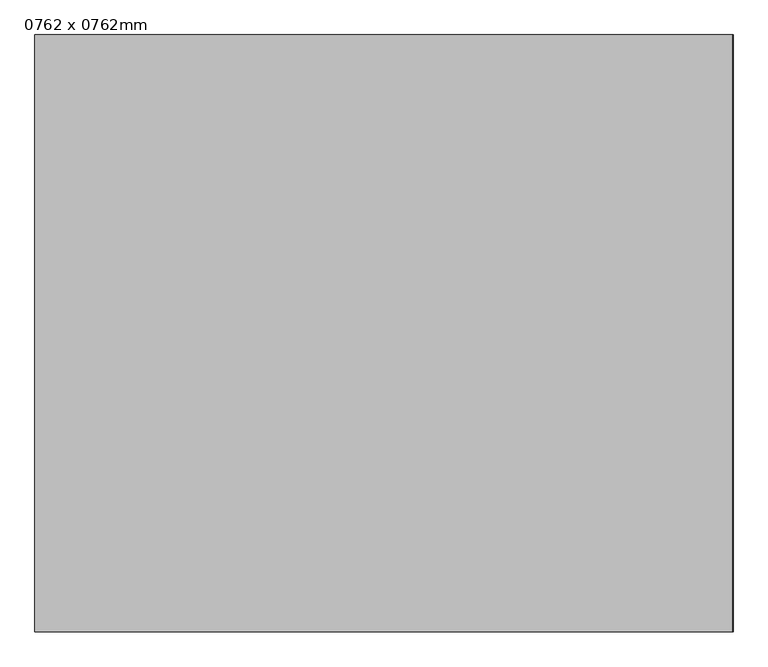
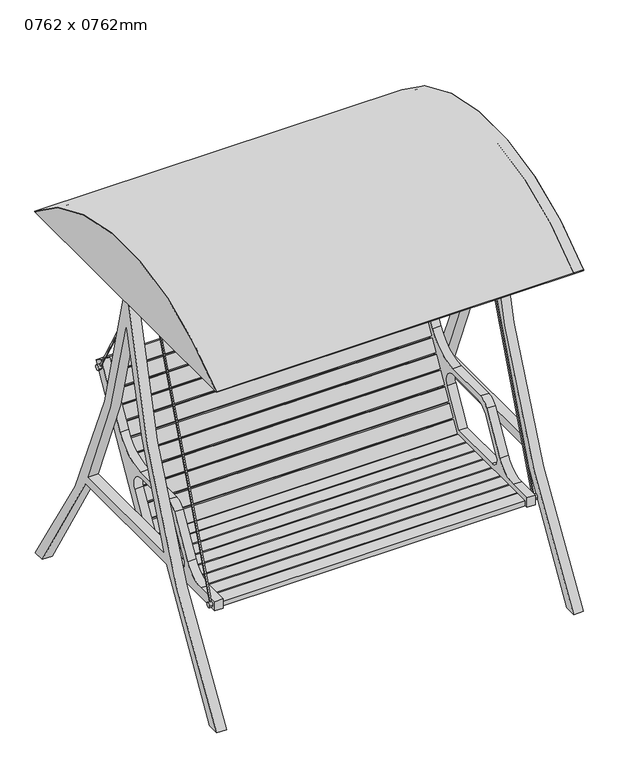
"""IFC4 building model written with IfcOpenShell, lengths in millimetres: furniture geometry, 0762 x 0762mm."""

from ifc_helpers import new_model, si_unit, point, frame, frame_2d, origin, place, context, project, spatial, polyline, circle_curve, trimmed, segment, composite_curve, outline, extrude, source, transform, mapped, element, save


def furniture_0762_x_0762mm_a8fad5e2(model_context):
    return source(origin(), model_context, "Body", "SweptSolid", [
        extrude(outline(composite_curve([segment(trimmed(circle_curve(frame_2d((4189.9023331, 1950.2809332)), 3303.1244251), [point((933.45, 1396.9734505))], [point((1524.0, 0.0))], True, "CARTESIAN"), True, "CONTINUOUS"), segment(polyline([(1524.0, 0.0), (1476.936255, 0.0)]), True, "CONTINUOUS"), segment(trimmed(circle_curve(frame_2d((4189.9023331, 1950.2809332)), 3341.2244251), [point((1476.936255, 0.0))], [point((1186.3373595, 486.5944542))], False, "CARTESIAN"), True, "CONTINUOUS"), segment(polyline([(1186.3373595, 486.5944542), (642.4626405, 486.5944542)]), True, "CONTINUOUS"), segment(trimmed(circle_curve(frame_2d((-2361.1023331, 1950.2809332)), 3341.2244251), [point((642.4626405, 486.5944542))], [point((351.863745, 0.0))], False, "CARTESIAN"), True, "CONTINUOUS"), segment(polyline([(351.863745, 0.0), (304.8, 0.0)]), True, "CONTINUOUS"), segment(trimmed(circle_curve(frame_2d((-2361.1023331, 1950.2809332)), 3303.1244251), [point((304.8, 0.0))], [point((895.35, 1396.9734505))], True, "CARTESIAN"), True, "CONTINUOUS"), segment(polyline([(895.35, 1396.9734505), (895.35, 1524.0), (914.4, 1524.0), (933.45, 1524.0), (933.45, 1396.9734505)]), True, "CONTINUOUS")], self_intersect=False), holes=[composite_curve([segment(polyline([(660.7321842, 524.6944542), (1168.0678158, 524.6944542)]), True, "CONTINUOUS"), segment(trimmed(circle_curve(frame_2d((4189.9023331, 1950.2809332)), 3341.2244251), [point((1168.0678158, 524.6944542))], [point((914.4, 1290.8378915))], False, "CARTESIAN"), True, "CONTINUOUS"), segment(trimmed(circle_curve(frame_2d((-2361.1023331, 1950.2809332)), 3341.2244251), [point((914.4, 1290.8378915))], [point((660.7321842, 524.6944542))], False, "CARTESIAN"), True, "CONTINUOUS")], self_intersect=False)]), frame((-272.362745, 0.0, 0.0), z_axis=(1.0, 0.0, 0.0), x_axis=(0.0, 1.0, 0.0)), (0.0, 0.0, 1.0), 38.1),
        extrude(outline(composite_curve([segment(trimmed(circle_curve(frame_2d((4189.9023331, 1950.2809332)), 3303.1244251), [point((933.45, 1396.9734505))], [point((1524.0, 0.0))], True, "CARTESIAN"), True, "CONTINUOUS"), segment(polyline([(1524.0, 0.0), (1476.936255, 0.0)]), True, "CONTINUOUS"), segment(trimmed(circle_curve(frame_2d((4189.9023331, 1950.2809332)), 3341.2244251), [point((1476.936255, 0.0))], [point((1186.3373595, 486.5944542))], False, "CARTESIAN"), True, "CONTINUOUS"), segment(polyline([(1186.3373595, 486.5944542), (642.4626405, 486.5944542)]), True, "CONTINUOUS"), segment(trimmed(circle_curve(frame_2d((-2361.1023331, 1950.2809332)), 3341.2244251), [point((642.4626405, 486.5944542))], [point((351.863745, 0.0))], False, "CARTESIAN"), True, "CONTINUOUS"), segment(polyline([(351.863745, 0.0), (304.8, 0.0)]), True, "CONTINUOUS"), segment(trimmed(circle_curve(frame_2d((-2361.1023331, 1950.2809332)), 3303.1244251), [point((304.8, 0.0))], [point((895.35, 1396.9734505))], True, "CARTESIAN"), True, "CONTINUOUS"), segment(polyline([(895.35, 1396.9734505), (895.35, 1524.0), (914.4, 1524.0), (933.45, 1524.0), (933.45, 1396.9734505)]), True, "CONTINUOUS")], self_intersect=False), holes=[composite_curve([segment(polyline([(660.7321842, 524.6944542), (1168.0678158, 524.6944542)]), True, "CONTINUOUS"), segment(trimmed(circle_curve(frame_2d((4189.9023331, 1950.2809332)), 3341.2244251), [point((1168.0678158, 524.6944542))], [point((914.4, 1290.8378915))], False, "CARTESIAN"), True, "CONTINUOUS"), segment(trimmed(circle_curve(frame_2d((-2361.1023331, 1950.2809332)), 3341.2244251), [point((914.4, 1290.8378915))], [point((660.7321842, 524.6944542))], False, "CARTESIAN"), True, "CONTINUOUS")], self_intersect=False)]), frame((1111.937255, 0.0, 0.0), z_axis=(1.0, 0.0, 0.0), x_axis=(0.0, 1.0, 0.0)), (0.0, 0.0, 1.0), 38.1),
        extrude(outline(polyline([(1111.937255, 933.45), (1111.937255, 895.35), (-234.262745, 895.35), (-234.262745, 933.45), (1111.937255, 933.45)])), frame((0.0, 0.0, 1484.1023899), z_axis=(0.0, 0.0, 1.0), x_axis=(1.0, 0.0, 0.0)), (0.0, 0.0, 1.0), 39.8976101),
        extrude(outline(composite_curve([segment(trimmed(circle_curve(frame_2d((914.4, 699.3747703)), 926.421113), [point((304.8, 1396.9734505))], [point((1524.0, 1396.9734505))], False, "CARTESIAN"), True, "CONTINUOUS"), segment(polyline([(1524.0, 1396.9734505), (304.8, 1396.9734505)]), True, "CONTINUOUS")], self_intersect=False), holes=[composite_curve([segment(polyline([(376.708681, 1422.3734505), (1452.091319, 1422.3734505)]), True, "CONTINUOUS"), segment(trimmed(circle_curve(frame_2d((914.4, 699.3747703)), 901.021113), [point((1452.091319, 1422.3734505))], [point((376.708681, 1422.3734505))], True, "CARTESIAN"), True, "CONTINUOUS")], self_intersect=False)]), frame((-272.362745, 0.0, 0.0), z_axis=(1.0, 0.0, 0.0), x_axis=(0.0, 1.0, 0.0)), (0.0, 0.0, 1.0), 38.1),
        extrude(outline(composite_curve([segment(trimmed(circle_curve(frame_2d((914.4, 699.3747703)), 926.421113), [point((304.8, 1396.9734505))], [point((1524.0, 1396.9734505))], False, "CARTESIAN"), True, "CONTINUOUS"), segment(polyline([(1524.0, 1396.9734505), (304.8, 1396.9734505)]), True, "CONTINUOUS")], self_intersect=False), holes=[composite_curve([segment(polyline([(376.708681, 1422.3734505), (1452.091319, 1422.3734505)]), True, "CONTINUOUS"), segment(trimmed(circle_curve(frame_2d((914.4, 699.3747703)), 901.021113), [point((1452.091319, 1422.3734505))], [point((376.708681, 1422.3734505))], True, "CARTESIAN"), True, "CONTINUOUS")], self_intersect=False)]), frame((1111.937255, 0.0, 0.0), z_axis=(1.0, 0.0, 0.0), x_axis=(0.0, 1.0, 0.0)), (0.0, 0.0, 1.0), 38.1),
        extrude(outline(composite_curve([segment(trimmed(circle_curve(frame_2d((914.4, 699.3747703)), 926.421113), [point((304.8, 1396.9734505))], [point((1524.0, 1396.9734505))], False, "CARTESIAN"), True, "CONTINUOUS"), segment(polyline([(1524.0, 1396.9734505), (304.8, 1396.9734505)]), True, "CONTINUOUS")], self_intersect=False)), frame((-273.952745, 0.0, 0.0), z_axis=(1.0, 0.0, 0.0), x_axis=(0.0, 1.0, 0.0)), (0.0, 0.0, 1.0), 1.59),
        extrude(outline(composite_curve([segment(trimmed(circle_curve(frame_2d((914.4, 699.3747703)), 926.421113), [point((304.8, 1396.9734505))], [point((1524.0, 1396.9734505))], False, "CARTESIAN"), True, "CONTINUOUS"), segment(polyline([(1524.0, 1396.9734505), (304.8, 1396.9734505)]), True, "CONTINUOUS")], self_intersect=False)), frame((1150.037255, 0.0, 0.0), z_axis=(1.0, 0.0, 0.0), x_axis=(0.0, 1.0, 0.0)), (0.0, 0.0, 1.0), 1.59),
        extrude(outline(composite_curve([segment(trimmed(circle_curve(frame_2d((914.4, 699.3747703)), 926.421113), [point((1524.0, 1396.9734505))], [point((304.8, 1396.9734505))], True, "CARTESIAN"), True, "CONTINUOUS"), segment(polyline([(304.8, 1396.9734505), (304.8, 1399.0836139)]), True, "CONTINUOUS"), segment(trimmed(circle_curve(frame_2d((914.4, 699.3747703)), 928.011113), [point((304.8, 1399.0836139))], [point((1524.0, 1399.0836139))], False, "CARTESIAN"), True, "CONTINUOUS"), segment(polyline([(1524.0, 1399.0836139), (1524.0, 1396.9734505)]), True, "CONTINUOUS")], self_intersect=False)), frame((-273.952745, 0.0, 0.0), z_axis=(1.0, 0.0, 0.0), x_axis=(0.0, 1.0, 0.0)), (0.0, 0.0, 1.0), 1423.99),
        extrude(outline(composite_curve([segment(trimmed(circle_curve(frame_2d((563.6419667, 511.4)), 105.0), [point((563.6419667, 406.4))], [point((654.5746341, 458.9))], True, "CARTESIAN"), True, "CONTINUOUS"), segment(polyline([(654.5746341, 458.9), (741.8122598, 610.0)]), True, "CONTINUOUS"), segment(trimmed(circle_curve(frame_2d((785.11353, 585.0)), 50.0), [point((741.8122598, 610.0))], [point((785.11353, 635.0))], False, "CARTESIAN"), True, "CONTINUOUS"), segment(polyline([(785.11353, 635.0), (968.6699734, 635.0)]), True, "CONTINUOUS"), segment(trimmed(circle_curve(frame_2d((968.6699734, 795.0)), 160.0), [point((968.6699734, 635.0))], [point((1107.2340381, 715.0))], True, "CARTESIAN"), True, "CONTINUOUS"), segment(polyline([(1107.2340381, 715.0), (1233.863745, 934.3290861), (1266.8593129, 915.2790861), (951.0607902, 368.3), (471.863745, 368.3), (471.863745, 406.4), (563.6419667, 406.4)]), True, "CONTINUOUS")], self_intersect=False), holes=[composite_curve([segment(trimmed(circle_curve(frame_2d((807.1413638, 546.8466726)), 62.7533274), [point((807.1413638, 609.6))], [point((752.7953881, 578.2233363))], True, "CARTESIAN"), True, "CONTINUOUS"), segment(polyline([(752.7953881, 578.2233363), (679.5739008, 451.4)]), True, "CONTINUOUS"), segment(trimmed(circle_curve(frame_2d((705.5546629, 436.4)), 30.0), [point((679.5739008, 451.4))], [point((705.5546629, 406.4))], True, "CARTESIAN"), True, "CONTINUOUS"), segment(polyline([(705.5546629, 406.4), (929.063745, 406.4), (1007.4101765, 542.1)]), True, "CONTINUOUS"), segment(trimmed(circle_curve(frame_2d((968.4390333, 564.6)), 45.0), [point((1007.4101765, 542.1))], [point((968.4390333, 609.6))], True, "CARTESIAN"), True, "CONTINUOUS"), segment(polyline([(968.4390333, 609.6), (807.1413638, 609.6)]), True, "CONTINUOUS")], self_intersect=False)]), frame((-184.03019, 0.0, 0.0), z_axis=(1.0, 0.0, 0.0), x_axis=(0.0, 1.0, 0.0)), (0.0, 0.0, 1.0), 32.5713093),
        extrude(outline(composite_curve([segment(trimmed(circle_curve(frame_2d((563.6419667, 511.4)), 105.0), [point((563.6419667, 406.4))], [point((654.5746341, 458.9))], True, "CARTESIAN"), True, "CONTINUOUS"), segment(polyline([(654.5746341, 458.9), (741.8122598, 610.0)]), True, "CONTINUOUS"), segment(trimmed(circle_curve(frame_2d((785.11353, 585.0)), 50.0), [point((741.8122598, 610.0))], [point((785.11353, 635.0))], False, "CARTESIAN"), True, "CONTINUOUS"), segment(polyline([(785.11353, 635.0), (968.6699734, 635.0)]), True, "CONTINUOUS"), segment(trimmed(circle_curve(frame_2d((968.6699734, 795.0)), 160.0), [point((968.6699734, 635.0))], [point((1107.2340381, 715.0))], True, "CARTESIAN"), True, "CONTINUOUS"), segment(polyline([(1107.2340381, 715.0), (1233.863745, 934.3290861), (1266.8593129, 915.2790861), (951.0607902, 368.3), (471.863745, 368.3), (471.863745, 406.4), (563.6419667, 406.4)]), True, "CONTINUOUS")], self_intersect=False), holes=[composite_curve([segment(trimmed(circle_curve(frame_2d((807.1413638, 546.8466726)), 62.7533274), [point((807.1413638, 609.6))], [point((752.7953881, 578.2233363))], True, "CARTESIAN"), True, "CONTINUOUS"), segment(polyline([(752.7953881, 578.2233363), (679.5739008, 451.4)]), True, "CONTINUOUS"), segment(trimmed(circle_curve(frame_2d((705.5546629, 436.4)), 30.0), [point((679.5739008, 451.4))], [point((705.5546629, 406.4))], True, "CARTESIAN"), True, "CONTINUOUS"), segment(polyline([(705.5546629, 406.4), (929.063745, 406.4), (1007.4101765, 542.1)]), True, "CONTINUOUS"), segment(trimmed(circle_curve(frame_2d((968.4390333, 564.6)), 45.0), [point((1007.4101765, 542.1))], [point((968.4390333, 609.6))], True, "CARTESIAN"), True, "CONTINUOUS"), segment(polyline([(968.4390333, 609.6), (807.1413638, 609.6)]), True, "CONTINUOUS")], self_intersect=False)]), frame((1027.5433908, 0.0, 0.0), z_axis=(1.0, 0.0, 0.0), x_axis=(0.0, 1.0, 0.0)), (0.0, 0.0, 1.0), 32.5713093),
        extrude(outline(polyline([(0.0, -19.0500001), (0.0, 0.0), (1179.0022715, 0.0), (1179.0022715, -19.0500001), (0.0, -19.0500001)])), frame((1027.5433908, 1224.9615289, 880.8099956), z_axis=(0.0, 0.5000000000000067, 0.8660254037844349), x_axis=(-1.0, 0.0, 0.0)), (0.0, 0.0, 1.0), 50.8),
        extrude(outline(polyline([(0.0, -19.0500001), (0.0, 0.0), (1179.0022715, 0.0), (1179.0022715, -19.0500001), (0.0, -19.0500001)])), frame((1027.5433908, 1196.3865289, 831.3166438), z_axis=(0.0, 0.5000000000000067, 0.8660254037844349), x_axis=(-1.0, 0.0, 0.0)), (0.0, 0.0, 1.0), 50.8),
        extrude(outline(polyline([(0.0, -19.0500001), (0.0, 0.0), (1179.0022715, 0.0), (1179.0022715, -19.0500001), (0.0, -19.0500001)])), frame((1027.5433908, 1167.8115289, 781.823292), z_axis=(0.0, 0.5000000000000067, 0.8660254037844349), x_axis=(-1.0, 0.0, 0.0)), (0.0, 0.0, 1.0), 50.8),
        extrude(outline(polyline([(0.0, -19.0500001), (0.0, 0.0), (1179.0022715, 0.0), (1179.0022715, -19.0500001), (0.0, -19.0500001)])), frame((1027.5433908, 1139.2365289, 732.3299402), z_axis=(0.0, 0.5000000000000067, 0.8660254037844349), x_axis=(-1.0, 0.0, 0.0)), (0.0, 0.0, 1.0), 50.8),
        extrude(outline(polyline([(0.0, -19.0500001), (0.0, 0.0), (1179.0022715, 0.0), (1179.0022715, -19.0500001), (0.0, -19.0500001)])), frame((1027.5433908, 1110.6615289, 682.8365883), z_axis=(0.0, 0.5000000000000067, 0.8660254037844349), x_axis=(-1.0, 0.0, 0.0)), (0.0, 0.0, 1.0), 50.8),
        extrude(outline(polyline([(0.0, -19.0500001), (0.0, 0.0), (1179.0022715, 0.0), (1179.0022715, -19.0500001), (0.0, -19.0500001)])), frame((1027.5433908, 1082.0865289, 633.3432365), z_axis=(0.0, 0.5000000000000067, 0.8660254037844349), x_axis=(-1.0, 0.0, 0.0)), (0.0, 0.0, 1.0), 50.8),
        extrude(outline(polyline([(0.0, -19.0500001), (0.0, 0.0), (1179.0022715, 0.0), (1179.0022715, -19.0500001), (0.0, -19.0500001)])), frame((1027.5433908, 1053.5115289, 583.8498847), z_axis=(0.0, 0.5000000000000067, 0.8660254037844349), x_axis=(-1.0, 0.0, 0.0)), (0.0, 0.0, 1.0), 50.8),
        extrude(outline(polyline([(0.0, -19.0500001), (0.0, 0.0), (1179.0022715, 0.0), (1179.0022715, -19.0500001), (0.0, -19.0500001)])), frame((1027.5433908, 1024.9365289, 534.3565329), z_axis=(0.0, 0.5000000000000067, 0.8660254037844349), x_axis=(-1.0, 0.0, 0.0)), (0.0, 0.0, 1.0), 50.8),
        extrude(outline(polyline([(0.0, -19.0500001), (0.0, 0.0), (1179.0022715, 0.0), (1179.0022715, -19.0500001), (0.0, -19.0500001)])), frame((1027.5433908, 996.3615289, 484.863181), z_axis=(0.0, 0.5000000000000067, 0.8660254037844349), x_axis=(-1.0, 0.0, 0.0)), (0.0, 0.0, 1.0), 50.8),
        extrude(outline(polyline([(0.0, -19.0500001), (0.0, 0.0), (1179.0022715, 0.0), (1179.0022715, -19.0500001), (0.0, -19.0500001)])), frame((1027.5433908, 967.7865289, 435.3698292), z_axis=(0.0, 0.5000000000000067, 0.8660254037844349), x_axis=(-1.0, 0.0, 0.0)), (0.0, 0.0, 1.0), 50.8),
        extrude(outline(polyline([(0.0, -19.0500001), (0.0, 0.0), (1179.0022715, 0.0), (1179.0022715, -19.0500001), (0.0, -19.0500001)])), frame((1027.5433908, 939.2115289, 385.8764774), z_axis=(0.0, 0.5000000000000067, 0.8660254037844349), x_axis=(-1.0, 0.0, 0.0)), (0.0, 0.0, 1.0), 50.8),
        extrude(outline(polyline([(1027.5433908, 933.8211), (1027.5433908, 883.0211), (-151.4588807, 883.0211), (-151.4588807, 933.8211), (1027.5433908, 933.8211)])), frame((0.0, 0.0, 368.3), z_axis=(0.0, 0.0, 1.0), x_axis=(1.0, 0.0, 0.0)), (0.0, 0.0, 1.0), 19.05),
        extrude(outline(polyline([(1027.5433908, 876.6711), (1027.5433908, 825.8711), (-151.4588807, 825.8711), (-151.4588807, 876.6711), (1027.5433908, 876.6711)])), frame((0.0, 0.0, 368.3), z_axis=(0.0, 0.0, 1.0), x_axis=(1.0, 0.0, 0.0)), (0.0, 0.0, 1.0), 19.05),
        extrude(outline(polyline([(1027.5433908, 819.5211), (1027.5433908, 768.7211), (-151.4588807, 768.7211), (-151.4588807, 819.5211), (1027.5433908, 819.5211)])), frame((0.0, 0.0, 368.3), z_axis=(0.0, 0.0, 1.0), x_axis=(1.0, 0.0, 0.0)), (0.0, 0.0, 1.0), 19.05),
        extrude(outline(polyline([(1027.5433908, 762.3711), (1027.5433908, 711.5711), (-151.4588807, 711.5711), (-151.4588807, 762.3711), (1027.5433908, 762.3711)])), frame((0.0, 0.0, 368.3), z_axis=(0.0, 0.0, 1.0), x_axis=(1.0, 0.0, 0.0)), (0.0, 0.0, 1.0), 19.05),
        extrude(outline(polyline([(1027.5433908, 705.2211), (1027.5433908, 654.4211), (-151.4588807, 654.4211), (-151.4588807, 705.2211), (1027.5433908, 705.2211)])), frame((0.0, 0.0, 368.3), z_axis=(0.0, 0.0, 1.0), x_axis=(1.0, 0.0, 0.0)), (0.0, 0.0, 1.0), 19.05),
        extrude(outline(polyline([(1027.5433908, 648.0711), (1027.5433908, 597.2711), (-151.4588807, 597.2711), (-151.4588807, 648.0711), (1027.5433908, 648.0711)])), frame((0.0, 0.0, 368.3), z_axis=(0.0, 0.0, 1.0), x_axis=(1.0, 0.0, 0.0)), (0.0, 0.0, 1.0), 19.05),
        extrude(outline(polyline([(1027.5433908, 590.9211), (1027.5433908, 540.1211), (-151.4588807, 540.1211), (-151.4588807, 590.9211), (1027.5433908, 590.9211)])), frame((0.0, 0.0, 368.3), z_axis=(0.0, 0.0, 1.0), x_axis=(1.0, 0.0, 0.0)), (0.0, 0.0, 1.0), 19.05),
        extrude(outline(polyline([(1027.5433908, 533.7711), (1027.5433908, 482.9711), (-151.4588807, 482.9711), (-151.4588807, 533.7711), (1027.5433908, 533.7711)])), frame((0.0, 0.0, 368.3), z_axis=(0.0, 0.0, 1.0), x_axis=(1.0, 0.0, 0.0)), (0.0, 0.0, 1.0), 19.05),
        extrude(outline(polyline([(914.4, 1484.1023899), (1241.1891484, 905.4891111), (1236.3748088, 902.7700689), (911.842017, 1477.3882398), (494.9813942, 383.2195737), (489.4362629, 385.3321793), (908.05, 1484.1023899), (914.4, 1484.1023899)])), frame((-188.7825876, 0.0, 0.0), z_axis=(1.0, 0.0, 0.0), x_axis=(0.0, 1.0, 0.0)), (0.0, 0.0, 1.0), 4.7523976),
        extrude(outline(composite_curve([segment(trimmed(circle_curve(frame_2d((1238.7819786, 904.12959)), 10.0), [point((1228.7819786, 904.12959))], [point((1248.7819786, 904.12959))], False, "CARTESIAN"), True, "CONTINUOUS"), segment(trimmed(circle_curve(frame_2d((1238.7819786, 904.12959)), 10.0), [point((1248.7819786, 904.12959))], [point((1228.7819786, 904.12959))], False, "CARTESIAN"), True, "CONTINUOUS")], self_intersect=False)), frame((-196.8218142, 0.0, 0.0), z_axis=(1.0, 0.0, 0.0), x_axis=(0.0, 1.0, 0.0)), (0.0, 0.0, 1.0), 12.7916242),
        extrude(outline(composite_curve([segment(trimmed(circle_curve(frame_2d((492.2088285, 384.2758765)), 10.0), [point((482.2088285, 384.2758765))], [point((502.2088285, 384.2758765))], False, "CARTESIAN"), True, "CONTINUOUS"), segment(trimmed(circle_curve(frame_2d((492.2088285, 384.2758765)), 10.0), [point((502.2088285, 384.2758765))], [point((482.2088285, 384.2758765))], False, "CARTESIAN"), True, "CONTINUOUS")], self_intersect=False)), frame((-196.8218142, 0.0, 0.0), z_axis=(1.0, 0.0, 0.0), x_axis=(0.0, 1.0, 0.0)), (0.0, 0.0, 1.0), 12.7916242),
        extrude(outline(polyline([(914.4, 1484.1023899), (1241.1891484, 905.4891111), (1236.3748088, 902.7700689), (911.842017, 1477.3882398), (494.9813942, 383.2195737), (489.4362629, 385.3321793), (908.05, 1484.1023899), (914.4, 1484.1023899)])), frame((1061.7047, 0.0, 0.0), z_axis=(1.0, 0.0, 0.0), x_axis=(0.0, 1.0, 0.0)), (0.0, 0.0, 1.0), 4.7523976),
        extrude(outline(composite_curve([segment(trimmed(circle_curve(frame_2d((1238.7819786, 904.12959)), 10.0), [point((1228.7819786, 904.12959))], [point((1248.7819786, 904.12959))], False, "CARTESIAN"), True, "CONTINUOUS"), segment(trimmed(circle_curve(frame_2d((1238.7819786, 904.12959)), 10.0), [point((1248.7819786, 904.12959))], [point((1228.7819786, 904.12959))], False, "CARTESIAN"), True, "CONTINUOUS")], self_intersect=False)), frame((1061.7047, 0.0, 0.0), z_axis=(1.0, 0.0, 0.0), x_axis=(0.0, 1.0, 0.0)), (0.0, 0.0, 1.0), 12.7916242),
        extrude(outline(composite_curve([segment(trimmed(circle_curve(frame_2d((492.2088285, 384.2758765)), 10.0), [point((482.2088285, 384.2758765))], [point((502.2088285, 384.2758765))], False, "CARTESIAN"), True, "CONTINUOUS"), segment(trimmed(circle_curve(frame_2d((492.2088285, 384.2758765)), 10.0), [point((502.2088285, 384.2758765))], [point((482.2088285, 384.2758765))], False, "CARTESIAN"), True, "CONTINUOUS")], self_intersect=False)), frame((1061.7047, 0.0, 0.0), z_axis=(1.0, 0.0, 0.0), x_axis=(0.0, 1.0, 0.0)), (0.0, 0.0, 1.0), 12.7916242),
    ])


if __name__ == "__main__":
    model = new_model("IFC4")
    model_context = context("Model", 3, world=origin())
    ifc_project = project(units=[si_unit("LENGTHUNIT", "METRE", prefix="MILLI")], contexts=[model_context])
    site = spatial("IfcSite", under=ifc_project)
    building = spatial("IfcBuilding", under=site)
    placement = place(None, origin())
    furniture_0762_x_0762mm_shape = furniture_0762_x_0762mm_a8fad5e2(model_context)
    element("IfcFurniture", 1, ObjectType="0762 x 0762mm", at=placement, inside=building, context=model_context, shape_type="MappedRepresentation", body=[
        mapped(furniture_0762_x_0762mm_shape, transform((0.0, 0.0, 0.0), x_axis=(1.0, 0.0, 0.0), y_axis=(0.0, 1.0, 0.0), z_axis=(0.0, 0.0, 1.0))),
    ])
    save(model, "model.ifc")

# Revit data of these elements
# Type "0762 x 0762mm"
#   Height = 1.499344 ft
#   Length = 2.5 ft
#   Width = 2.5 ft
#   Base Material = Wood - Birch
#   Top Material = Laminate - Ivory, Matte
#   Default Elevation = 0
# Element 1 (IfcFurniture, "0762 x 0762mm")
#   Materials on its faces: "wood finish", "steel", "Laminate - Ivory, Matte", "fabric"
# Materials
#   "Wood - Birch": class "Wood", colour RGB 224 178 126, transparency 0
#   "Laminate - Ivory, Matte": colour RGB 247 247 239, transparency 0
#   "wood finish": class "Generic", colour RGB 120 120 120, transparency 0, Cost = 0
#   "steel": class "Generic", colour RGB 120 120 120, transparency 0, Cost = 0
#   "fabric": class "Generic", colour RGB 120 120 120, transparency 0, Cost = 0
